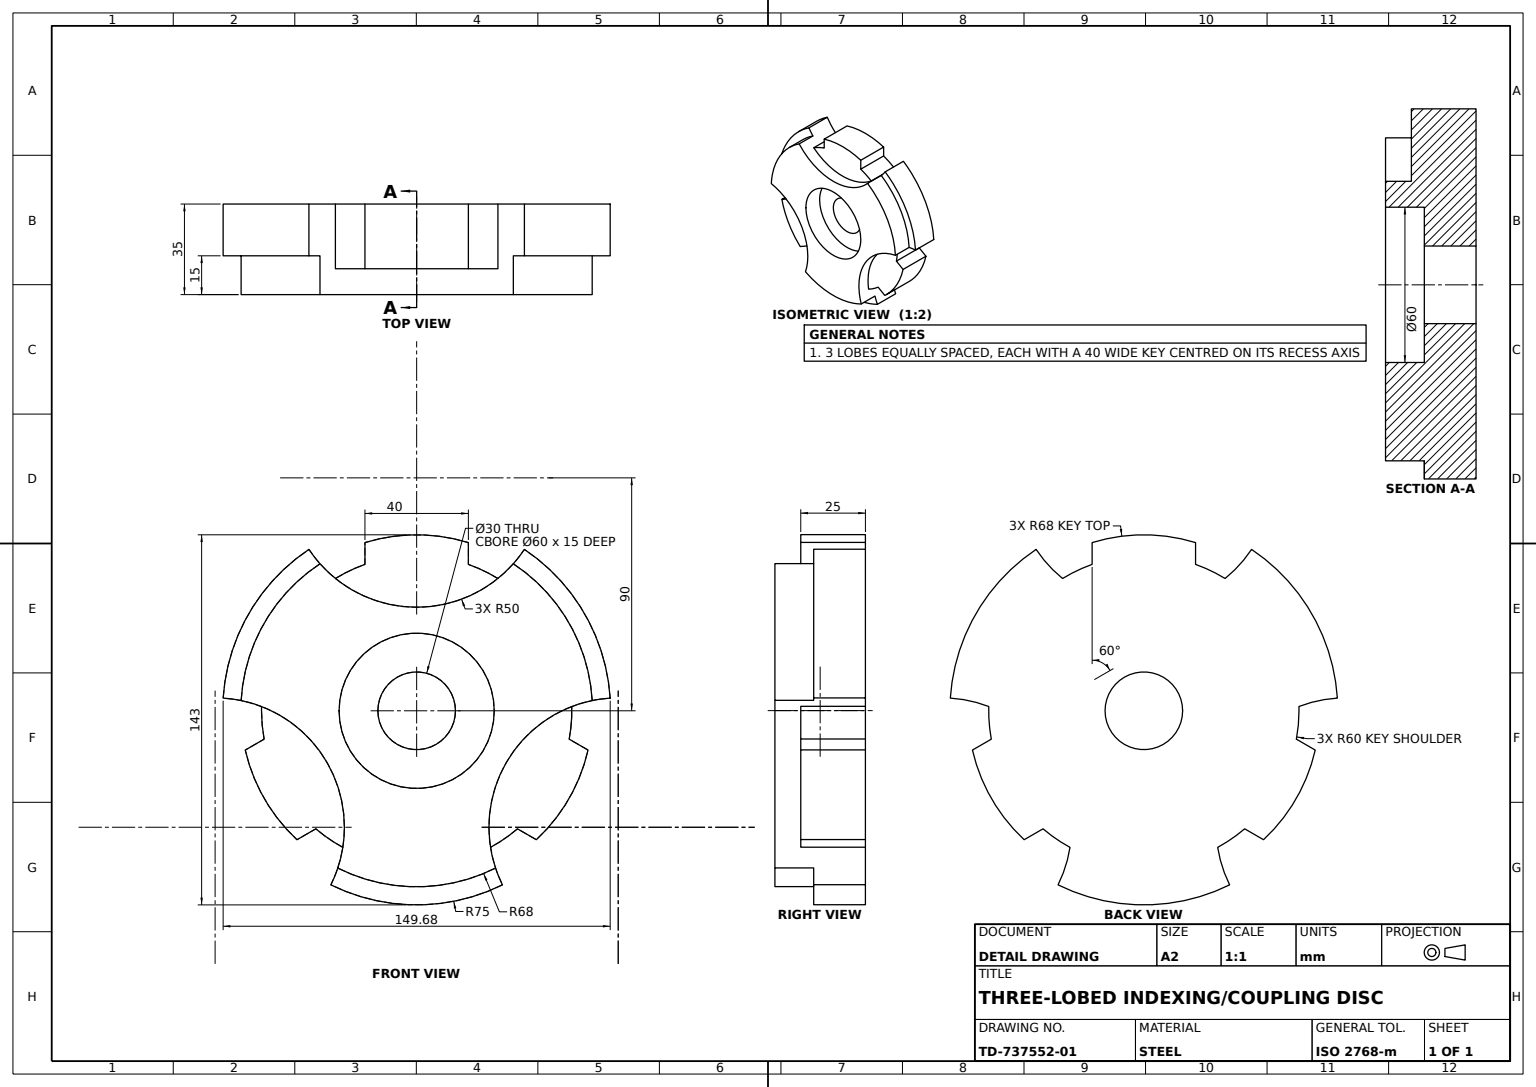
from build123d import *

# Parameters (mm, degrees)
BASE_DISC_SKETCH_R    = 75
BASE_DISC_DEPTH       = 20
HUB_BOSS_SKETCH_R     = 68
HUB_BOSS_DEPTH        = 15
LOBE_START            = -35
LOBE_RECESS_CUT_DEPTH = 35
COUPLING_LOBES_DEPTH  = 25
COUNTERBORE_SKETCH_R  = 30
COUNTERBORE_DEPTH     = 15
THROUGH_BORE_SKETCH_R = 15
THROUGH_BORE_DEPTH    = 20


with BuildPart() as part:
    # Base Disc Sketch → Base Disc (new body)
    with BuildSketch(Plane.XY):
        Circle(BASE_DISC_SKETCH_R)
    extrude(amount=BASE_DISC_DEPTH)

    # Hub Boss Sketch → Hub Boss (add)
    with BuildSketch(Plane.XY.offset(20)):
        Circle(HUB_BOSS_SKETCH_R)
    extrude(amount=HUB_BOSS_DEPTH)

    # Lobe Recess Sketch → Lobe Recess Cut (cut)
    with BuildSketch(Plane.XY.offset(35).offset(LOBE_START)):
        with BuildLine():
            ThreePointArc((-37.386628626, 56.8), (-19.514097468, 65.139849555), (0, 68))
            Line((0, 68), (0, 90))
            ThreePointArc((0, 90), (-25, 86.458082329), (-48.032267961, 76.111111111))
            ThreePointArc((-48.032267961, 76.111111111), (-43.787289555, 65.861373829), (-37.386628626, 56.8))
        make_face()
        with BuildLine():
            Line((0, 90), (0, 68))
            ThreePointArc((0, 68), (19.514097468, 65.139849555), (37.386628626, 56.8))
            ThreePointArc((37.386628626, 56.8), (43.787289555, 65.861373829), (48.032267961, 76.111111111))
            ThreePointArc((48.032267961, 76.111111111), (25, 86.458082329), (0, 90))
        make_face()
        with BuildLine():
            ThreePointArc((-37.386628626, 56.8), (-20.493901532, 44.392982996), (0, 40))
            Line((0, 40), (0, 68))
            ThreePointArc((0, 68), (-19.514097468, 65.139849555), (-37.386628626, 56.8))
        make_face()
        with BuildLine():
            Line((0, 68), (0, 40))
            ThreePointArc((0, 40), (20.493901532, 44.392982996), (37.386628626, 56.8))
            ThreePointArc((37.386628626, 56.8), (19.514097468, 65.139849555), (0, 68))
        make_face()
        with BuildLine():
            ThreePointArc((58.889727457, -34), (46.655715779, -49.469628917), (30.496928622, -60.777770152))
            ThreePointArc((30.496928622, -60.777770152), (35.143978087, -70.851592032), (41.898021752, -79.652719811))
            ThreePointArc((41.898021752, -79.652719811), (62.374895659, -64.879676259), (77.942286341, -45))
            Line((77.942286341, -45), (58.889727457, -34))
        make_face()
        with BuildLine():
            ThreePointArc((67.883557248, 3.977770152), (67.970883078, 1.989737061), (68, 0))
            ThreePointArc((68, 0), (65.682956188, -17.599695067), (58.889727457, -34))
            Line((58.889727457, -34), (77.942286341, -45))
            ThreePointArc((77.942286341, -45), (86.933324366, -23.293714059), (90, 0))
            ThreePointArc((90, 0), (89.982570741, 1.771147347), (89.930289713, 3.5416087))
            ThreePointArc((89.930289713, 3.5416087), (78.931267642, 4.990218203), (67.883557248, 3.977770152))
        make_face()
        with BuildLine():
            Line((68, 0), (56.147791623, 0))
            ThreePointArc((56.147791623, 0), (43.892842113, -8.385312403), (34.641016151, -20))
            Line((34.641016151, -20), (58.889727457, -34))
            ThreePointArc((58.889727457, -34), (65.682956188, -17.599695067), (68, 0))
        make_face()
        with BuildLine():
            Line((58.889727457, -34), (34.641016151, -20))
            ThreePointArc((34.641016151, -20), (28.198500258, -39.944730847), (30.496928622, -60.777770152))
            ThreePointArc((30.496928622, -60.777770152), (46.655715779, -49.469628917), (58.889727457, -34))
        make_face()
        with BuildLine():
            ThreePointArc((67.883557248, 3.977770152), (61.891970748, 2.353852741), (56.147791623, 0))
            Line((56.147791623, 0), (68, 0))
            ThreePointArc((68, 0), (67.970883078, 1.989737061), (67.883557248, 3.977770152))
        make_face()
        with BuildLine():
            ThreePointArc((-41.898021752, -79.652719811), (-35.143978087, -70.851592032), (-30.496928622, -60.777770152))
            ThreePointArc((-30.496928622, -60.777770152), (-46.655715779, -49.469628917), (-58.889727457, -34))
            Line((-58.889727457, -34), (-77.942286341, -45))
            ThreePointArc((-77.942286341, -45), (-62.374895659, -64.879676259), (-41.898021752, -79.652719811))
        make_face()
        with BuildLine():
            ThreePointArc((-58.889727457, -34), (-65.682956188, -17.599695067), (-68, 0))
            ThreePointArc((-68, 0), (-67.970883078, 1.989737061), (-67.883557248, 3.977770152))
            ThreePointArc((-67.883557248, 3.977770152), (-78.931267642, 4.990218203), (-89.930289713, 3.5416087))
            ThreePointArc((-89.930289713, 3.5416087), (-87.374895659, -21.57840607), (-77.942286341, -45))
            Line((-77.942286341, -45), (-58.889727457, -34))
        make_face()
        with BuildLine():
            ThreePointArc((-34.641016151, -20), (-43.892842113, -8.385312403), (-56.147791623, 0))
            Line((-56.147791623, 0), (-68, 0))
            ThreePointArc((-68, 0), (-65.682956188, -17.599695067), (-58.889727457, -34))
            Line((-58.889727457, -34), (-34.641016151, -20))
        make_face()
        with BuildLine():
            ThreePointArc((-27.942286341, -45), (-29.645995026, -32.059047745), (-34.641016151, -20))
            Line((-34.641016151, -20), (-58.889727457, -34))
            ThreePointArc((-58.889727457, -34), (-46.655715779, -49.469628917), (-30.496928622, -60.777770152))
            ThreePointArc((-30.496928622, -60.777770152), (-28.585078732, -52.99162418), (-27.942286341, -45))
        make_face()
        with BuildLine():
            Line((-68, 0), (-56.147791623, 0))
            ThreePointArc((-56.147791623, 0), (-61.891970748, 2.353852741), (-67.883557248, 3.977770152))
            ThreePointArc((-67.883557248, 3.977770152), (-67.970883078, 1.989737061), (-68, 0))
        make_face()
    extrude(amount=LOBE_RECESS_CUT_DEPTH, mode=Mode.SUBTRACT)

    # Coupling Lobes Sketch → Coupling Lobes (add)
    with BuildSketch(Plane(origin=(0, 0, 0), x_dir=(-1, 0, 0), z_dir=(0, 0, -1))):
        with BuildLine():
            ThreePointArc((-31.426968053, 51.111111111), (-16.666666667, 42.859547921), (0, 40))
            Line((0, 40), (0, 68))
            ThreePointArc((0, 68), (-10.112445497, 67.243872926), (-20, 64.992307237))
            Line((-20, 64.992307237), (-20, 56.568542495))
            ThreePointArc((-20, 56.568542495), (-25.857864376, 54.142135624), (-31.426968053, 51.111111111))
        make_face()
        with BuildLine():
            Line((0, 68), (0, 40))
            ThreePointArc((0, 40), (16.666666667, 42.859547921), (31.426968053, 51.111111111))
            ThreePointArc((31.426968053, 51.111111111), (25.857864376, 54.142135624), (20, 56.568542495))
            Line((20, 56.568542495), (20, 64.992307237))
            ThreePointArc((20, 64.992307237), (10.112445497, 67.243872926), (0, 68))
        make_face()
        with BuildLine():
            Line((-46.284989118, -49.816661694), (-38.989794856, -45.604779323))
            ThreePointArc((-38.989794856, -45.604779323), (-33.959532677, -49.464635249), (-28.550036612, -52.772108253))
            ThreePointArc((-28.550036612, -52.772108253), (-34.641016151, -20), (-59.977004664, 1.660997142))
            ThreePointArc((-59.977004664, 1.660997142), (-59.817397053, -4.677500374), (-58.989794856, -10.963763172))
            Line((-58.989794856, -10.963763172), (-66.284989118, -15.175645543))
            ThreePointArc((-66.284989118, -15.175645543), (-58.889727457, -34), (-46.284989118, -49.816661694))
        make_face()
        with BuildLine():
            Line((66.284989118, -15.175645543), (58.989794856, -10.963763172))
            ThreePointArc((58.989794856, -10.963763172), (59.817397053, -4.677500374), (59.977004664, 1.660997142))
            ThreePointArc((59.977004664, 1.660997142), (34.641016151, -20), (28.550036612, -52.772108253))
            ThreePointArc((28.550036612, -52.772108253), (33.959532677, -49.464635249), (38.989794856, -45.604779323))
            Line((38.989794856, -45.604779323), (46.284989118, -49.816661694))
            ThreePointArc((46.284989118, -49.816661694), (58.889727457, -34), (66.284989118, -15.175645543))
        make_face()
    extrude(amount=-COUPLING_LOBES_DEPTH)

    # Counterbore Sketch → Counterbore (cut)
    with BuildSketch(Plane.XY.offset(35)):
        Circle(COUNTERBORE_SKETCH_R)
    extrude(amount=-COUNTERBORE_DEPTH, mode=Mode.SUBTRACT)

    # Through Bore Sketch → Through Bore (cut)
    with BuildSketch(Plane.XY.offset(20)):
        Circle(THROUGH_BORE_SKETCH_R)
    extrude(amount=-THROUGH_BORE_DEPTH, mode=Mode.SUBTRACT)


solid = part.part
